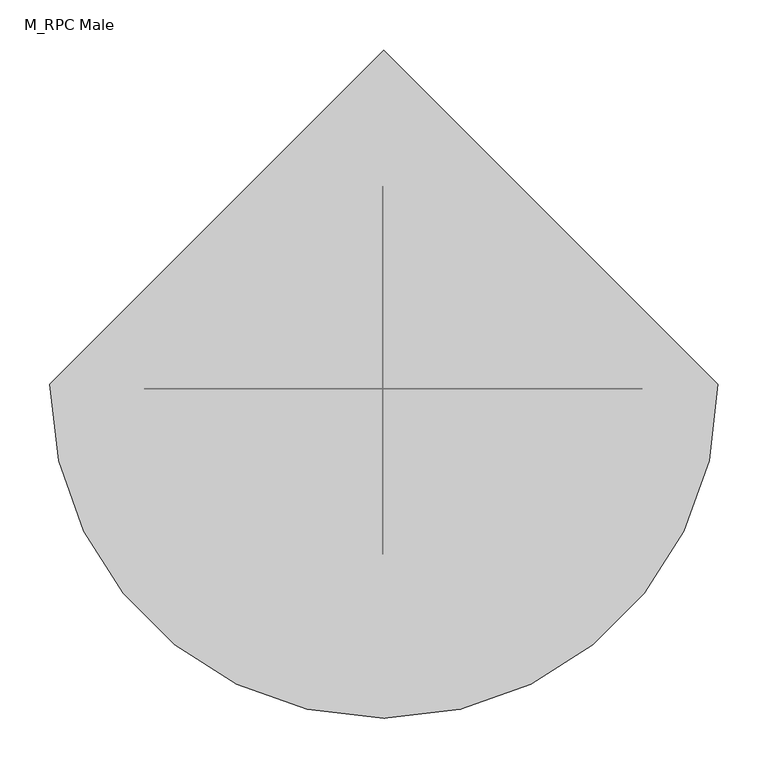
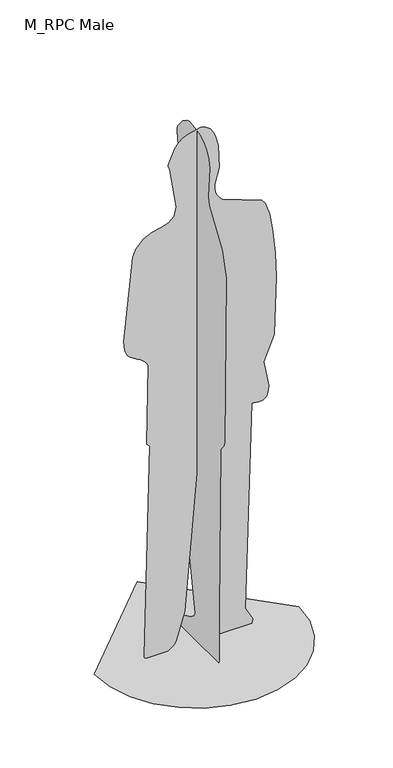
"""IFC4 building model written with IfcOpenShell, lengths in millimetres: proxy geometry, M_RPC Male."""

from ifc_helpers import new_model, si_unit, origin, place, context, project, spatial, triangles, source, transform, mapped, element, save


def m_rpc_male_90c61d85(model_context):
    return source(origin(), model_context, "Body", "Tessellation", [
        triangles([(-180.7520848, -4.45e-05, 5.61e-05), (-184.2428783, -8.8e-06, 2.7953159), (-186.1722845, 1.66e-05, 5.8375037), (-186.8317464, 3.35e-05, 9.1275735), (-168.2847136, 8.5e-06, 733.0655743), (-173.8813923, 8.5e-06, 735.2245268), (-177.6699692, 8.1e-06, 740.933626), (-174.1986331, -8.1e-06, 1013.6688681), (-179.5913999, -8.8e-06, 1024.1657564), (-188.0396306, -9.6e-06, 1032.776568), (-198.5268175, -9.9e-06, 1040.1131115), (-210.0364347, -1.03e-05, 1046.7870501), (-221.5521744, -1.07e-05, 1053.4098289), (-232.0573471, -1.1e-05, 1060.5935474), (-240.5355178, -1.14e-05, 1068.9494328), (-245.9520113, -1.21e-05, 1078.9886456), (-249.738826, -1.29e-05, 1091.9828379), (-252.1553936, -1.4e-05, 1106.9305447), (-253.4609098, -1.47e-05, 1122.8302282), (-224.2189811, -3.16e-05, 1405.0553707), (-213.7950534, -3.31e-05, 1430.202673), (-189.1320602, -3.46e-05, 1456.0851048), (-160.6250248, -3.53e-05, 1468.8744404), (-131.9230613, -3.57e-05, 1475.6385624), (-106.6753564, -3.64e-05, 1483.4444813), (-88.5310696, -3.71e-05, 1499.3602249), (-81.1393152, -3.9e-05, 1530.4523678), (-102.9420995, -4.71e-05, 1666.4706642), (-107.9472991, -4.78e-05, 1679.2659588), (-108.1475049, -4.82e-05, 1680.5750359), (-107.9848786, -4.82e-05, 1682.7597862), (-107.5268942, -4.82e-05, 1685.5199375), (-106.8410076, -4.86e-05, 1688.5562347), (-86.6409506, -5.11e-05, 1733.0913071), (-74.2774702, -5.19e-05, 1747.7193386), (-59.5121923, -5.26e-05, 1759.6604702), (-42.3631437, -5.33e-05, 1768.7786636), (-0.985526, -5.37e-05, 1778.0000484), (15.8808848, -5.33e-05, 1772.5537239), (29.1619713, -5.26e-05, 1761.5648598), (39.2640596, -5.19e-05, 1747.0972836), (46.5934905, -5.08e-05, 1731.2151134), (56.0091903, -4.89e-05, 1695.7216404), (59.1639804, -4.41e-05, 1618.2096565), (44.4858566, -4.12e-05, 1564.728764), (44.3096955, -4.05e-05, 1551.1871487), (46.5533085, -3.94e-05, 1537.928801), (51.2886617, -3.86e-05, 1525.4368309), (58.5876893, -3.83e-05, 1514.1934765), (68.5223527, -3.75e-05, 1504.6817024), (198.4031332, -3.46e-05, 1454.5815628), (210.7096676, -3.38e-05, 1440.8303673), (224.9006982, -3.13e-05, 1397.845491), (235.5370584, -2.72e-05, 1333.6076969), (242.7581838, -2.28e-05, 1256.1539944), (246.7033826, -1.77e-05, 1173.5217562), (240.2782843, -5.9e-06, 974.9295176), (206.0814981, -1.1e-06, 891.6227566), (221.1963095, 4e-06, 805.6637592), (220.4651768, 5.1e-06, 788.6204681), (214.9949983, 6.3e-06, 771.8049248), (210.3553106, 6.6e-06, 765.7305136), (204.1669347, 6.6e-06, 762.0922909), (196.8960849, 7e-06, 760.3985716), (189.0091026, 7e-06, 760.1578159), (180.9722204, 7e-06, 760.8779028), (173.2516706, 6.6e-06, 762.0673651), (166.3136674, 6.6e-06, 763.2342997), (144.8011906, 4.49e-05, 59.4753214), (168.627625, 4.74e-05, 15.3365923), (166.1986854, -4.45e-05, 5.61e-05), (66.1332407, -4.45e-05, 5.61e-05), (49.8425291, -1.03e-05, 3.9765611), (39.0246438, 1.36e-05, 14.0353079), (32.5983191, 2.91e-05, 28.3297275), (-2.744106, 9.2e-06, 720.0463108), (-54.0725352, 1.03e-05, 117.9433913), (-81.3720589, -2.13e-05, 28.0047564), (-85.5237496, -2.69e-05, 19.9172799), (-91.2434313, -3.27e-05, 12.569124), (-99.2451958, -3.86e-05, 5.9378916), (-110.2432618, -4.45e-05, 5.61e-05), (-13.8237486, -127.6719491, 9.9621202), (-13.8238042, -127.2618269, 182.0843436), (-13.8237883, -135.2636459, 744.8699409), (-13.8237883, -136.4150655, 748.3464729), (-13.8237883, -139.3955431, 752.5740492), (-13.8237883, -143.4944753, 757.5063063), (-13.8237883, -148.0011678, 763.0967354), (-13.8237883, -152.2050719, 769.2988277), (-13.8237872, -155.3954567, 776.0660746), (-13.8237872, -156.8617008, 783.3521124), (-13.823769, -165.9465932, 1358.6144554), (-13.8237679, -143.2744033, 1442.0935169), (-13.8237645, -71.1145909, 1552.8594303), (-13.8237645, -64.3402088, 1580.52155), (-13.823761, -73.5344423, 1684.7962898), (-13.823761, -67.2131576, 1712.2171452), (-13.823761, -55.2412502, 1734.9080566), (-13.823761, -37.9260417, 1752.7547871), (-13.823761, -15.5748862, 1765.6435352), (-13.823761, 11.5049141, 1773.4603546), (-13.823761, 43.0060141, 1776.0911533), (-13.823761, 55.0860544, 1772.9173645), (-13.823761, 79.7039013, 1756.3228832), (-13.8237633, 107.489678, 1722.3487942), (-13.8237633, 111.5712331, 1713.0111374), (-13.8237633, 112.222992, 1702.3027794), (-13.8237667, 99.083278, 1611.9293713), (-13.8237667, 100.6007817, 1597.8215115), (-13.8237679, 96.7552315, 1579.0665516), (-13.823769, 31.1784725, 1488.4601635), (-13.8237803, 125.7984987, 1146.7478817), (-13.8237803, 134.1994394, 1137.675761), (-13.8237826, 184.2799945, 1119.3931561), (-13.8237826, 194.4650741, 1111.9401226), (-13.8237826, 201.1344345, 1100.3807264), (-13.8237838, 203.5509657, 1084.206423), (-13.8237838, 200.9675115, 1068.9646208), (-13.8237838, 194.2821819, 1055.8713066), (-13.8237838, 184.3929236, 1046.142104), (-13.8237838, 172.1979013, 1040.9932903), (-13.8237838, 158.5950979, 1041.6404892), (-13.8237838, 144.4825418, 1049.2996874), (-13.8237917, 123.0430165, 785.7652645), (-13.8237928, 116.9063816, 707.2433132), (-13.8237997, 10.2023739, 90.6853713), (-13.8238019, 17.9839052, 76.1482317), (-13.8238031, 35.4714586, 63.8067748), (-13.8238121, 104.5965861, 31.8661645), (-13.8238133, 119.3345037, 20.2173774), (-13.8238144, 122.9915752, 6.7192125), (-13.8238121, 122.0607817, 4.3675023), (-13.8237974, 120.3452342, 2.3141491), (-13.8237803, 119.1854304, 1.4285661), (-13.8237542, 117.8200068, 0.6534774), (-13.8237179, 116.2459023, 5.61e-05), (-13.8237145, -124.5016756, 0.0), (-348.4736423, 4.7230064, 0.0001684), (-339.5989297, -72.1961928, 0.0001684), (-314.32391, -142.8341776, 5.61e-05), (-274.6723695, -205.1670917, 5.61e-05), (-222.6682945, -257.1712212, 5.61e-05), (-160.335326, -296.8226708, 5.61e-05), (-89.6973593, -322.0977087, 5.61e-05), (-12.7781717, -330.9724214, 5.61e-05), (64.1410249, -322.097745, 5.61e-05), (134.7790098, -296.8227253, 5.61e-05), (197.1119329, -257.171203, 5.61e-05), (249.1161169, -205.167128, 5.61e-05), (288.7675302, -142.8341322, 5.61e-05), (314.0425681, -72.1961337, 0.0001684), (322.9173171, 4.7230357, 0.0001684), (-12.7782308, 340.4184291, 0.0001684)], [[70, 71, 72], [69, 70, 72], [69, 72, 73], [69, 73, 74], [69, 74, 75], [69, 75, 76], [68, 69, 76], [82, 1, 2], [82, 2, 3], [82, 3, 4], [81, 82, 4], [80, 81, 4], [79, 80, 4], [78, 79, 4], [77, 78, 4], [77, 4, 5], [76, 77, 5], [5, 6, 7], [76, 5, 7], [76, 7, 8], [68, 76, 8], [67, 68, 8], [66, 67, 8], [65, 66, 8], [64, 65, 8], [63, 64, 8], [62, 63, 8], [61, 62, 8], [60, 61, 8], [59, 60, 8], [58, 59, 8], [57, 58, 8], [56, 57, 8], [56, 8, 9], [55, 56, 9], [55, 9, 10], [54, 55, 10], [54, 10, 11], [53, 54, 11], [53, 11, 12], [52, 53, 12], [51, 52, 12], [50, 51, 12], [50, 12, 13], [50, 13, 14], [50, 14, 15], [50, 15, 16], [50, 16, 17], [50, 17, 18], [50, 18, 19], [50, 19, 20], [50, 20, 21], [50, 21, 22], [50, 22, 23], [50, 23, 24], [50, 24, 25], [50, 25, 26], [49, 50, 26], [48, 49, 26], [48, 26, 27], [47, 48, 27], [46, 47, 27], [45, 46, 27], [44, 45, 27], [44, 27, 28], [43, 44, 28], [42, 43, 28], [42, 28, 29], [42, 29, 30], [42, 30, 31], [42, 31, 32], [42, 32, 33], [42, 33, 34], [42, 34, 35], [42, 35, 36], [42, 36, 37], [41, 42, 37], [40, 41, 37], [40, 37, 38], [40, 38, 39], [137, 138, 83], [137, 83, 84], [136, 137, 84], [135, 136, 84], [130, 131, 132], [130, 132, 133], [130, 133, 134], [130, 134, 135], [122, 123, 124], [121, 122, 124], [120, 121, 124], [119, 120, 124], [118, 119, 124], [117, 118, 124], [116, 117, 124], [115, 116, 124], [114, 115, 124], [113, 114, 124], [106, 107, 108], [105, 106, 108], [104, 105, 108], [103, 104, 108], [102, 103, 108], [101, 102, 108], [100, 101, 108], [99, 100, 108], [98, 99, 108], [97, 98, 108], [97, 108, 109], [97, 109, 110], [97, 110, 111], [96, 97, 111], [95, 96, 111], [95, 111, 112], [94, 95, 112], [93, 94, 112], [93, 112, 113], [92, 93, 113], [92, 113, 124], [92, 124, 125], [91, 92, 125], [90, 91, 125], [89, 90, 125], [88, 89, 125], [87, 88, 125], [86, 87, 125], [86, 125, 126], [85, 86, 126], [85, 126, 127], [84, 85, 127], [84, 127, 128], [135, 84, 128], [135, 128, 129], [130, 135, 129], [153, 154, 139], [152, 153, 139], [152, 139, 140], [151, 152, 140], [151, 140, 141], [151, 141, 142], [150, 151, 142], [149, 150, 142], [149, 142, 143], [149, 143, 144], [149, 144, 145], [149, 145, 146], [149, 146, 147], [149, 147, 148]], closed=False),
    ])


if __name__ == "__main__":
    model = new_model("IFC4")
    model_context = context("Model", 3, world=origin())
    ifc_project = project(units=[si_unit("LENGTHUNIT", "METRE", prefix="MILLI")], contexts=[model_context])
    site = spatial("IfcSite", under=ifc_project)
    building = spatial("IfcBuilding", under=site)
    placement = place(None, origin())
    m_rpc_male_shape = m_rpc_male_90c61d85(model_context)
    element("IfcBuildingElementProxy", 1, Name="M_RPC Male", ObjectType="M_RPC Male", at=placement, inside=building, context=model_context, shape_type="MappedRepresentation", body=[
        mapped(m_rpc_male_shape, transform((0.0, 0.0, 0.0), x_axis=(1.0, 0.0, 0.0), y_axis=(0.0, 1.0, 0.0), z_axis=(0.0, 0.0, 1.0))),
    ])
    save(model, "model.ifc")

# Revit data of these elements
# Type "M_RPC Male"
#   built-in parameter 1005195 = "RPC-8-G1AE-S4G0-CKUK-A"
#   Height = 0
